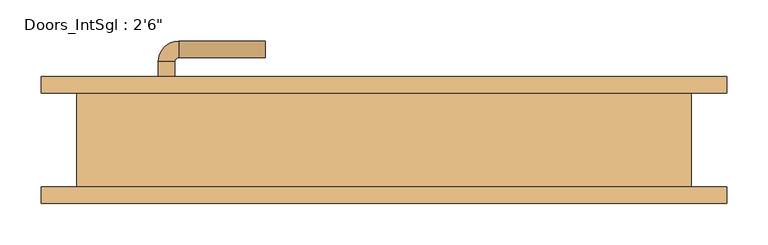
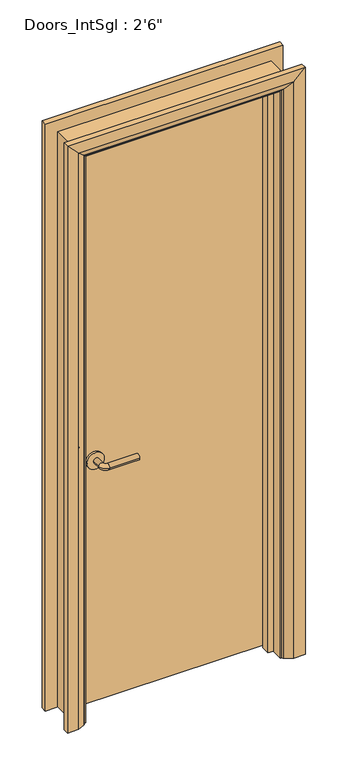
"""IFC4 building model written with IfcOpenShell, lengths in millimetres: door geometry."""

from ifc_helpers import new_model, si_unit, point, frame, frame_2d, origin, place, context, project, spatial, polyline, circle_curve, ellipse_curve, trimmed, segment, composite_curve, outline, extrude, faceted_brep, source, transform, mapped, element, save
from ifc_brep_helpers import plane_surface, cylinder_surface, revolved_surface, advanced_brep


def door_4bb05ab8(model_context):
    return source(origin(), model_context, "Body", "SolidModel", [
        advanced_brep(
        [(-274.0, 11.15, 900.0), (-254.0, 11.15, 900.0), (-254.0, -18.85, 900.0), (-274.0, -18.85, 900.0), (-249.0, -23.85, 900.0), (-249.0, -43.85, 900.0), (-144.0, -43.85, 900.0), (-144.0, -23.85, 900.0)],
        [
            (0, 1, circle_curve(frame((-264.0, 11.15, 900.0), z_axis=(0.0, 1.0, 0.0), x_axis=(1.0, 0.0, 0.0)), 10.0)),
            (1, 0, circle_curve(frame((-264.0, 11.15, 900.0), z_axis=(0.0, 1.0, 0.0), x_axis=(1.0, 0.0, 0.0)), 10.0)),
            (1, 2),
            (2, 3, circle_curve(frame((-264.0, -18.85, 900.0), z_axis=(0.0, 1.0, 0.0), x_axis=(1.0, 0.0, 0.0)), 10.0)),
            (3, 0),
            (3, 2, circle_curve(frame((-264.0, -18.85, 900.0), z_axis=(0.0, 1.0, 0.0), x_axis=(1.0, 0.0, 0.0)), 10.0)),
            (4, 5, circle_curve(frame((-249.0, -33.85, 900.0), z_axis=(-1.0, 0.0, 0.0), x_axis=(0.0, 1.0, 0.0)), 10.0)),
            (5, 3, circle_curve(frame((-249.0, -18.85, 900.0), z_axis=(0.0, 0.0, -1.0), x_axis=(-1.0, 0.0, 0.0)), 25.0)),
            (2, 4, circle_curve(frame((-249.0, -18.85, 900.0), z_axis=(0.0, 0.0, 1.0), x_axis=(-1.0, 0.0, 0.0)), 5.0)),
            (5, 4, circle_curve(frame((-249.0, -33.85, 900.0), z_axis=(-1.0, 0.0, 0.0), x_axis=(0.0, 1.0, 0.0)), 10.0)),
            (6, 7, circle_curve(frame((-144.0, -33.85, 900.0), z_axis=(1.0, 0.0, 0.0), x_axis=(0.0, 1.0, 0.0)), 10.0)),
            (7, 6, circle_curve(frame((-144.0, -33.85, 900.0), z_axis=(1.0, 0.0, 0.0), x_axis=(0.0, 1.0, 0.0)), 10.0)),
            (4, 7),
            (6, 5),
        ],
        [
            plane_surface(frame((-264.0, 11.15, 900.0), z_axis=(0.0, 1.0, 0.0), x_axis=(0.0, 0.0, 1.0))),
            cylinder_surface(frame((-264.0, 11.15, 900.0), z_axis=(0.0, 1.0, 0.0), x_axis=(1.0, 0.0, 0.0)), 10.0),
            revolved_surface(trimmed(ellipse_curve(frame((-264.0, -18.85, 900.0), z_axis=(0.0, -1.0, 0.0), x_axis=(1.0, 0.0, 0.0)), 10.0, 10.0), [point((-274.0, -18.85, 900.0))], [point((-254.0, -18.85, 900.0))], True, "CARTESIAN"), (-249.0, -18.85, 900.0), (0.0, 0.0, -1.0)),
            revolved_surface(trimmed(ellipse_curve(frame((-264.0, -18.85, 900.0), z_axis=(0.0, -1.0, 0.0), x_axis=(1.0, 0.0, 0.0)), 10.0, 10.0), [point((-254.0, -18.85, 900.0))], [point((-274.0, -18.85, 900.0))], True, "CARTESIAN"), (-249.0, -18.85, 900.0), (0.0, 0.0, -1.0)),
            plane_surface(frame((-144.0, -33.85, 900.0), z_axis=(1.0, 0.0, 0.0), x_axis=(0.0, 0.0, 1.0))),
            cylinder_surface(frame((-249.0, -33.85, 900.0), z_axis=(-1.0, 0.0, 0.0), x_axis=(0.0, 1.0, 0.0)), 10.0),
        ],
        [
            (0, [[1, 2]]),
            (1, [[3, 4, 5, -2]]),
            (1, [[-5, 6, -3, -1]]),
            (2, [[7, 8, -4, 9]]),
            (3, [[10, -9, -6, -8]]),
            (4, [[11, 12]]),
            (5, [[13, -11, 14, -7]]),
            (5, [[-14, -12, -13, -10]]),
        ],
    ),
        extrude(outline(composite_curve([segment(trimmed(circle_curve(frame_2d((900.0, -266.5)), 30.0), [point((900.0, -296.5))], [point((900.0, -236.5))], False, "CARTESIAN"), True, "CONTINUOUS"), segment(trimmed(circle_curve(frame_2d((900.0, -266.5)), 30.0), [point((900.0, -236.5))], [point((900.0, -296.5))], False, "CARTESIAN"), True, "CONTINUOUS")], self_intersect=False)), frame((0.0, 11.15, 0.0), z_axis=(0.0, 1.0, 0.0), x_axis=(0.0, 0.0, 1.0)), (0.0, 0.0, 1.0), 8.0),
        advanced_brep(
        [(-274.0, 65.15, 900.0), (-254.0, 65.15, 900.0), (-274.0, 95.15, 900.0), (-254.0, 95.15, 900.0), (-249.0, 100.15, 900.0), (-249.0, 120.15, 900.0), (-144.0, 120.15, 900.0), (-144.0, 100.15, 900.0)],
        [
            (0, 1, circle_curve(frame((-264.0, 65.15, 900.0), z_axis=(0.0, -1.0, 0.0), x_axis=(1.0, 0.0, 0.0)), 10.0)),
            (1, 0, circle_curve(frame((-264.0, 65.15, 900.0), z_axis=(0.0, -1.0, 0.0), x_axis=(1.0, 0.0, 0.0)), 10.0)),
            (0, 2),
            (2, 3, circle_curve(frame((-264.0, 95.15, 900.0), z_axis=(0.0, -1.0, 0.0), x_axis=(1.0, 0.0, 0.0)), 10.0)),
            (3, 1),
            (3, 2, circle_curve(frame((-264.0, 95.15, 900.0), z_axis=(0.0, -1.0, 0.0), x_axis=(1.0, 0.0, 0.0)), 10.0)),
            (4, 3, circle_curve(frame((-249.0, 95.15, 900.0), z_axis=(0.0, 0.0, 1.0), x_axis=(-1.0, 0.0, 0.0)), 5.0)),
            (2, 5, circle_curve(frame((-249.0, 95.15, 900.0), z_axis=(0.0, 0.0, -1.0), x_axis=(-1.0, 0.0, 0.0)), 25.0)),
            (5, 4, circle_curve(frame((-249.0, 110.15, 900.0), z_axis=(-1.0, 0.0, 0.0), x_axis=(0.0, -1.0, 0.0)), 10.0)),
            (4, 5, circle_curve(frame((-249.0, 110.15, 900.0), z_axis=(-1.0, 0.0, 0.0), x_axis=(0.0, -1.0, 0.0)), 10.0)),
            (6, 7, circle_curve(frame((-144.0, 110.15, 900.0), z_axis=(1.0, 0.0, 0.0), x_axis=(0.0, -1.0, 0.0)), 10.0)),
            (7, 6, circle_curve(frame((-144.0, 110.15, 900.0), z_axis=(1.0, 0.0, 0.0), x_axis=(0.0, -1.0, 0.0)), 10.0)),
            (5, 6),
            (7, 4),
        ],
        [
            plane_surface(frame((-264.0, 65.15, 900.0), z_axis=(0.0, -1.0, 0.0), x_axis=(0.0, 0.0, 1.0))),
            cylinder_surface(frame((-264.0, 65.15, 900.0), z_axis=(0.0, -1.0, 0.0), x_axis=(1.0, 0.0, 0.0)), 10.0),
            revolved_surface(trimmed(ellipse_curve(frame((-264.0, 95.15, 900.0), z_axis=(0.0, -1.0, 0.0), x_axis=(1.0, 0.0, 0.0)), 10.0, 10.0), [point((-274.0, 95.15, 900.0))], [point((-254.0, 95.15, 900.0))], True, "CARTESIAN"), (-249.0, 95.15, 900.0), (0.0, 0.0, -1.0)),
            revolved_surface(trimmed(ellipse_curve(frame((-264.0, 95.15, 900.0), z_axis=(0.0, -1.0, 0.0), x_axis=(1.0, 0.0, 0.0)), 10.0, 10.0), [point((-254.0, 95.15, 900.0))], [point((-274.0, 95.15, 900.0))], True, "CARTESIAN"), (-249.0, 95.15, 900.0), (0.0, 0.0, -1.0)),
            plane_surface(frame((-144.0, 110.15, 900.0), z_axis=(1.0, 0.0, 0.0), x_axis=(0.0, 0.0, 1.0))),
            cylinder_surface(frame((-249.0, 110.15, 900.0), z_axis=(-1.0, 0.0, 0.0), x_axis=(0.0, -1.0, 0.0)), 10.0),
        ],
        [
            (0, [[1, 2]]),
            (1, [[-1, 3, 4, 5]]),
            (1, [[-2, -5, 6, -3]]),
            (2, [[7, -4, 8, 9]]),
            (3, [[-8, -6, -7, 10]]),
            (4, [[11, 12]]),
            (5, [[-9, 13, -12, 14]]),
            (5, [[-10, -14, -11, -13]]),
        ],
    ),
        extrude(outline(composite_curve([segment(trimmed(circle_curve(frame_2d((900.0, -266.5)), 30.0), [point((900.0, -296.5))], [point((900.0, -236.5))], False, "CARTESIAN"), True, "CONTINUOUS"), segment(trimmed(circle_curve(frame_2d((900.0, -266.5)), 30.0), [point((900.0, -236.5))], [point((900.0, -296.5))], False, "CARTESIAN"), True, "CONTINUOUS")], self_intersect=False)), frame((0.0, 57.15, 0.0), z_axis=(0.0, 1.0, 0.0), x_axis=(0.0, 0.0, 1.0)), (0.0, 0.0, 1.0), 8.0),
        extrude(outline(polyline([(339.0, 19.15), (-339.0, 19.15), (-339.0, 57.15), (339.0, 57.15), (339.0, 19.15)])), frame((0.0, 0.0, 8.0), z_axis=(0.0, 0.0, 1.0), x_axis=(1.0, 0.0, 0.0)), (0.0, 0.0, 1.0), 2083.6),
        advanced_brep(
        [(416.0, 77.15, 0.0), (416.0, 57.15, 0.0), (346.0, 57.15, 0.0), (350.0, 63.15, 0.0), (376.0, 77.15, 0.0), (416.0, 77.15, 2168.6), (416.0, 57.15, 2168.6), (-416.0, 57.15, 2168.6), (-416.0, 57.15, 0.0), (-346.0, 57.15, 0.0), (-346.0, 57.15, 2098.6), (346.0, 57.15, 2098.6), (350.0, 63.15, 2102.6), (376.0, 77.15, 2128.6), (-376.0, 77.15, 2128.6), (-376.0, 77.15, 0.0), (-416.0, 77.15, 0.0), (-416.0, 77.15, 2168.6), (-350.0, 63.15, 0.0), (-350.0, 63.15, 2102.6)],
        [
            (0, 1),
            (1, 2),
            (2, 3, circle_curve(frame((354.0, 56.15, 0.0), z_axis=(0.0, 0.0, -1.0), x_axis=(1.0, 0.0, 0.0)), 8.0622577)),
            (3, 4),
            (4, 0),
            (0, 5),
            (5, 6),
            (6, 1),
            (6, 7),
            (7, 8),
            (8, 9),
            (9, 10),
            (10, 11),
            (11, 2),
            (11, 12, ellipse_curve(frame((354.0, 56.15, 2106.6), z_axis=(0.7071067811865475, 0.0, -0.7071067811865475), x_axis=(-0.7071067811865474, 0.0, -0.7071067811865476)), 11.4017543, 8.0622577)),
            (12, 3),
            (12, 13),
            (13, 4),
            (13, 14),
            (14, 15),
            (15, 16),
            (16, 17),
            (17, 5),
            (7, 17),
            (16, 8),
            (15, 18),
            (18, 9, circle_curve(frame((-354.0, 56.15, 0.0), z_axis=(0.0, 0.0, -1.0), x_axis=(-1.0, 0.0, 0.0)), 8.0622577)),
            (19, 10, ellipse_curve(frame((-354.0, 56.15, 2106.6), z_axis=(-0.7071067811865475, 0.0, -0.7071067811865475), x_axis=(-0.7071067811865474, 0.0, 0.7071067811865476)), 11.4017543, 8.0622577)),
            (18, 19),
            (14, 19),
            (19, 12),
        ],
        [
            plane_surface(frame((346.0, 57.15, 0.0), z_axis=(0.0, 0.0, -1.0), x_axis=(0.0, -1.0, 0.0))),
            plane_surface(frame((416.0, 77.15, 0.0), z_axis=(1.0, 0.0, 0.0), x_axis=(0.0, 0.0, 1.0))),
            plane_surface(frame((416.0, 57.15, 0.0), z_axis=(0.0, -1.0, 0.0), x_axis=(0.0, 0.0, 1.0))),
            cylinder_surface(frame((354.0, 56.15, 0.0), z_axis=(0.0, 0.0, -1.0), x_axis=(1.0, 0.0, 0.0)), 8.0622577),
            plane_surface(frame((350.0, 63.15, 0.0), z_axis=(-0.4740998230350126, 0.880471099922178, 0.0), x_axis=(0.0, 0.0, 1.0))),
            plane_surface(frame((376.0, 77.15, 0.0), z_axis=(0.0, 1.0, 0.0), x_axis=(0.0, 0.0, 1.0))),
            plane_surface(frame((-416.0, 77.15, 2168.6), z_axis=(-1.0, 0.0, 0.0), x_axis=(0.0, 0.0, -1.0))),
            plane_surface(frame((-346.0, 57.15, 0.0), z_axis=(0.0, 0.0, -1.0), x_axis=(0.0, -1.0, 0.0))),
            cylinder_surface(frame((-354.0, 56.15, 2098.6), z_axis=(0.0, 0.0, 1.0), x_axis=(-1.0, 0.0, 0.0)), 8.0622577),
            plane_surface(frame((-350.0, 63.15, 2102.6), z_axis=(0.47409982303501824, 0.8804710999221749, 0.0), x_axis=(0.0, 0.0, -1.0))),
            plane_surface(frame((416.0, 77.15, 2168.6), z_axis=(0.0, 0.0, 1.0), x_axis=(-1.0, 0.0, 0.0))),
            cylinder_surface(frame((346.0, 56.15, 2106.6), z_axis=(1.0, 0.0, 0.0), x_axis=(0.0, 0.0, 1.0)), 8.0622577),
            plane_surface(frame((350.0, 63.15, 2102.6), z_axis=(0.0, 0.8804710999221764, -0.4740998230350154), x_axis=(-1.0, 0.0, 0.0))),
        ],
        [
            (0, [[1, 2, 3, 4, 5]]),
            (1, [[-1, 6, 7, 8]]),
            (2, [[-2, -8, 9, 10, 11, 12, 13, 14]]),
            (3, [[-3, -14, 15, 16]]),
            (4, [[-4, -16, 17, 18]]),
            (5, [[-5, -18, 19, 20, 21, 22, 23, -6]]),
            (6, [[24, -22, 25, -10]]),
            (7, [[-21, 26, 27, -11, -25]]),
            (8, [[28, -12, -27, 29]]),
            (9, [[30, -29, -26, -20]]),
            (10, [[-7, -23, -24, -9]]),
            (11, [[-15, -13, -28, 31]]),
            (12, [[-17, -31, -30, -19]]),
        ],
    ),
        extrude(outline(polyline([(0.0, -341.0), (0.0, -322.0), (2074.6, -322.0), (2074.6, 322.0), (0.0, 322.0), (0.0, 341.0), (2093.6, 341.0), (2093.6, -341.0), (0.0, -341.0)])), frame((0.0, -14.85, 0.0), z_axis=(0.0, 1.0, 0.0), x_axis=(0.0, 0.0, 1.0)), (0.0, 0.0, 1.0), 32.0),
        advanced_brep(
        [(-416.0, -77.15, 0.0), (-416.0, -57.15, 0.0), (-346.0, -57.15, 0.0), (-350.0, -63.15, 0.0), (-376.0, -77.15, 0.0), (-416.0, -77.15, 2168.6), (-416.0, -57.15, 2168.6), (-346.0, -57.15, 2098.6), (-350.0, -63.15, 2102.6), (-376.0, -77.15, 2128.6), (416.0, -77.15, 0.0), (376.0, -77.15, 0.0), (350.0, -63.15, 0.0), (346.0, -57.15, 0.0), (416.0, -57.15, 0.0), (416.0, -77.15, 2168.6), (376.0, -77.15, 2128.6), (350.0, -63.15, 2102.6), (346.0, -57.15, 2098.6), (416.0, -57.15, 2168.6)],
        [
            (0, 1),
            (1, 2),
            (2, 3, circle_curve(frame((-354.0, -56.15, 0.0), z_axis=(0.0, 0.0, -1.0), x_axis=(-1.0, 0.0, 0.0)), 8.0622577)),
            (3, 4),
            (4, 0),
            (0, 5),
            (5, 6),
            (6, 1),
            (6, 7),
            (7, 2),
            (7, 8, ellipse_curve(frame((-354.0, -56.15, 2106.6), z_axis=(-0.7071067811865475, 0.0, -0.7071067811865475), x_axis=(0.7071067811865474, 0.0, -0.7071067811865476)), 11.4017543, 8.0622577)),
            (8, 3),
            (8, 9),
            (9, 4),
            (9, 5),
            (10, 11),
            (11, 12),
            (12, 13, circle_curve(frame((354.0, -56.15, 0.0), z_axis=(0.0, 0.0, -1.0), x_axis=(1.0, 0.0, 0.0)), 8.0622577)),
            (13, 14),
            (14, 10),
            (15, 16),
            (16, 11),
            (10, 15),
            (16, 17),
            (17, 12),
            (17, 18, ellipse_curve(frame((354.0, -56.15, 2106.6), z_axis=(0.7071067811865475, 0.0, -0.7071067811865475), x_axis=(0.7071067811865474, 0.0, 0.7071067811865476)), 11.4017543, 8.0622577)),
            (18, 13),
            (18, 19),
            (19, 14),
            (19, 15),
            (5, 15),
            (19, 6),
            (18, 7),
            (17, 8),
            (16, 9),
        ],
        [
            plane_surface(frame((-346.0, -129.9510989, 0.0), z_axis=(0.0, 0.0, -1.0), x_axis=(1.0, 0.0, 0.0))),
            plane_surface(frame((-416.0, -77.15, 0.0), z_axis=(-1.0, 0.0, 0.0), x_axis=(0.0, 0.0, 1.0))),
            plane_surface(frame((-416.0, -57.15, 0.0), z_axis=(0.0, 1.0, 0.0), x_axis=(0.0, 0.0, 1.0))),
            cylinder_surface(frame((-354.0, -56.15, 0.0), z_axis=(0.0, 0.0, -1.0), x_axis=(-1.0, 0.0, 0.0)), 8.0622577),
            plane_surface(frame((-350.0, -63.15, 0.0), z_axis=(0.4740998230350183, -0.8804710999221749, 0.0), x_axis=(0.0, 0.0, 1.0))),
            plane_surface(frame((-376.0, -77.15, 0.0), z_axis=(0.0, -1.0, 0.0), x_axis=(0.0, 0.0, 1.0))),
            plane_surface(frame((346.0, -129.9510989, 0.0), z_axis=(0.0, 0.0, -1.0), x_axis=(-1.0, 0.0, 0.0))),
            plane_surface(frame((376.0, -77.15, 2128.6), z_axis=(0.0, -1.0, 0.0), x_axis=(0.0, 0.0, -1.0))),
            plane_surface(frame((350.0, -63.15, 2102.6), z_axis=(-0.4740998230350183, -0.8804710999221749, 0.0), x_axis=(0.0, 0.0, -1.0))),
            cylinder_surface(frame((354.0, -56.15, 2098.6), z_axis=(0.0, 0.0, 1.0), x_axis=(1.0, 0.0, 0.0)), 8.0622577),
            plane_surface(frame((416.0, -57.15, 2168.6), z_axis=(0.0, 1.0, 0.0), x_axis=(0.0, 0.0, -1.0))),
            plane_surface(frame((416.0, -77.15, 2168.6), z_axis=(1.0, 0.0, 0.0), x_axis=(0.0, 0.0, -1.0))),
            plane_surface(frame((-416.0, -77.15, 2168.6), z_axis=(0.0, 0.0, 1.0), x_axis=(1.0, 0.0, 0.0))),
            plane_surface(frame((-416.0, -57.15, 2168.6), z_axis=(0.0, 1.0, 0.0), x_axis=(1.0, 0.0, 0.0))),
            cylinder_surface(frame((-346.0, -56.15, 2106.6), z_axis=(-1.0, 0.0, 0.0), x_axis=(0.0, 0.0, 1.0)), 8.0622577),
            plane_surface(frame((-350.0, -63.15, 2102.6), z_axis=(0.0, -0.8804710999221749, -0.4740998230350183), x_axis=(1.0, 0.0, 0.0))),
            plane_surface(frame((-376.0, -77.15, 2128.6), z_axis=(0.0, -1.0, 0.0), x_axis=(1.0, 0.0, 0.0))),
        ],
        [
            (0, [[1, 2, 3, 4, 5]]),
            (1, [[-1, 6, 7, 8]]),
            (2, [[-2, -8, 9, 10]]),
            (3, [[-3, -10, 11, 12]]),
            (4, [[-4, -12, 13, 14]]),
            (5, [[-5, -14, 15, -6]]),
            (6, [[16, 17, 18, 19, 20]]),
            (7, [[21, 22, -16, 23]]),
            (8, [[24, 25, -17, -22]]),
            (9, [[26, 27, -18, -25]]),
            (10, [[28, 29, -19, -27]]),
            (11, [[30, -23, -20, -29]]),
            (12, [[-7, 31, -30, 32]]),
            (13, [[-9, -32, -28, 33]]),
            (14, [[-11, -33, -26, 34]]),
            (15, [[-13, -34, -24, 35]]),
            (16, [[-15, -35, -21, -31]]),
        ],
    ),
        faceted_brep([(-341.0, 57.15, 0.0), (-341.0, -57.15, 0.0), (-373.0, -57.15, 0.0), (-373.0, 57.15, 0.0), (-341.0, 57.15, 2093.6), (-341.0, -57.15, 2093.6), (-373.0, -57.15, 2125.6), (-373.0, 57.15, 2125.6), (341.0, 57.15, 0.0), (373.0, 57.15, 0.0), (373.0, -57.15, 0.0), (341.0, -57.15, 0.0), (341.0, 57.15, 2093.6), (373.0, 57.15, 2125.6), (373.0, -57.15, 2125.6), (341.0, -57.15, 2093.6)], [[[0, 1, 2, 3]], [[1, 0, 4, 5]], [[2, 1, 5, 6]], [[3, 2, 6, 7]], [[0, 3, 7, 4]], [[8, 9, 10, 11]], [[12, 13, 9, 8]], [[13, 14, 10, 9]], [[14, 15, 11, 10]], [[15, 12, 8, 11]], [[5, 4, 12, 15]], [[6, 5, 15, 14]], [[7, 6, 14, 13]], [[4, 7, 13, 12]]]),
    ])


if __name__ == "__main__":
    model = new_model("IFC4")
    model_context = context("Model", 3, world=origin())
    ifc_project = project(units=[si_unit("LENGTHUNIT", "METRE", prefix="MILLI")], contexts=[model_context])
    site = spatial("IfcSite", under=ifc_project)
    building = spatial("IfcBuilding", under=site)
    placement = place(None, origin())
    door_shape = door_4bb05ab8(model_context)
    element("IfcDoor", 1, ObjectType="Doors_IntSgl : 2'6\"", at=placement, inside=building, context=model_context, shape_type="MappedRepresentation", body=[
        mapped(door_shape, transform((0.0, 0.0, 0.0), x_axis=(1.0, 0.0, 0.0), y_axis=(0.0, 1.0, 0.0), z_axis=(0.0, 0.0, 1.0))),
    ])
    save(model, "model.ifc")

# Revit data of these elements
# Type "Doors_IntSgl : 2'6\""
#   Type Mark = "48"
#   Type Comments = "Internal Single"
#   Operation = "SingleSwingRight"
#   Manufacturer = "Revit"
#   Keynote = "L20"
#   Description = "Internal Single Door"
#   Analytic Construction = "Metal"
#   UnderCut = 0' - 0.31496"
#   Tolerance = 0' - 0.07874"
#   Thickness = 0' - 1.49606"
#   Thermal Resistance (R) = 0.270117 (m²·K)/W
#   Structural Tolerance = 0' - 0.31496"
#   StopDepth = 0' - 1.25984"
#   Stop Thickness = 0' - 0.74803"
#   Rough Width = 2' - 6"
#   Rough Height = 7' - 0"
#   Height to Top Lock Rail = 3' - 3.37008"
#   Heat Transfer Coefficient (U) = 3.7021 W/(m²·K)
#   Handle Z Distance = 2' - 11.43307"
#   Handle X Distance = 0' - 2.95276"
#   Frame Thickness = 0' - 1.25984"
#   Door Panel Width = 2' - 2.69291"
#   Door Panel Thickness = 0' - 1.49606"
#   Door Panel Offset = 0' - 0"
#   Height = 7' - 0"
#   Width = 2' - 6"
#   Door Panel Height = 6' - 10.0315"
#   Architrave Setback = 0' - 0.19685"
#   Vis - Ironmongery = yes
#   Material Ironmongery = Door - Handle
#   Material Frame = Door - Frame/Mullion (1)
#   Material Door = Door - Panel
#   Material Architrave = Door - Architrave
#   Visual Light Transmittance = 0
#   Solar Heat Gain Coefficient = 0
#   Function = (empty or 0)
#   Wall Closure = (empty or 0)
# Element 1 (IfcDoor, "Doors_IntSgl : 2'6\"")
#   Materials on its faces: "Door - Architrave", "Door - Handle", "Door - Frame/Mullion (1)", "Door - Panel"
# Materials
#   "Door - Handle": colour RGB 0 0 0, transparency 0, Keynote = "P21", Cost = 0
#   "Door - Frame/Mullion (1)": class "Wood", colour RGB 212 179 113, transparency 0, Keynote = "L20", Cost = 0
#   "Door - Panel": class "Wood", colour RGB 210 159 95, transparency 0, Keynote = "L20", Cost = 0
#   "Door - Architrave": class "Wood", colour RGB 154 90 5, transparency 0, Keynote = "P20", Cost = 0
